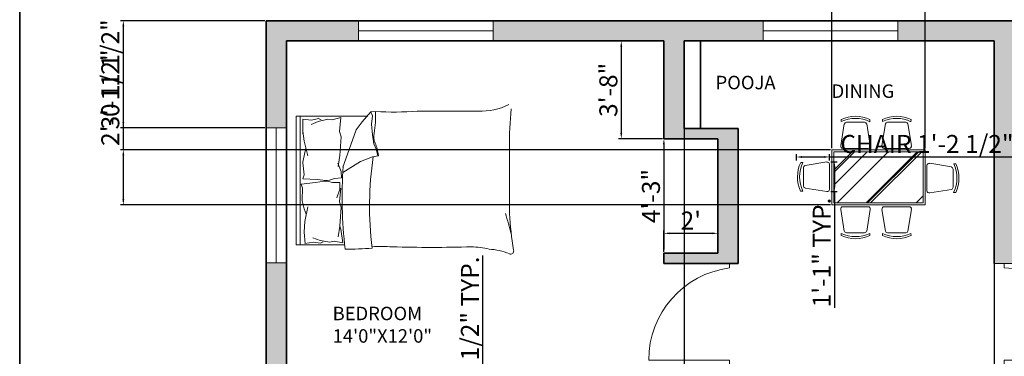
# Model space of a CAD drawing. Units: inches. Extents: x 2257 to 3678, y 834 to 1975.
# Tile 4 of 16: x 2257 to 2696, y 1444 to 1594. Entities that reach past the tile are written whole.
import ezdxf

# ---------------------------------------------------------------- set-up
doc = ezdxf.new("R2010")
doc.units = ezdxf.units.IN
for name, color, linetype, lineweight in [('A-ANNO-DIMS', 2, 'Continuous', 18), ('A-ANNO-TTLB', 7, 'Continuous', 35), ('A-AREA-IDEN', 7, 'Continuous', 18), ('A-DOOR', 3, 'Continuous', 18), ('A-FURN', 8, 'Continuous', 18), ('A-FURN-PATT', 8, 'Continuous', 13), ('A-GLAZ', 4, 'Continuous', 18), ('A-WALL', 7, 'Continuous', 35)]:
    doc.layers.add(name, color=color, linetype=linetype, lineweight=lineweight)
doc.layers.add('A-WALL-PATT', color=251, linetype='Continuous', lineweight=13, true_color=0x636466)
doc.styles.get("Standard").update_dxf_attribs({"font": 'arial.ttf'})
doc.dimstyles.new('ISO-25', dxfattribs={"dimtxt": 8, "dimasz": 2.5, "dimexe": 1.25, "dimexo": 0.625, "dimtad": 1, "dimdec": 0, "dimlunit": 3, "dimtxsty": 'Standard', "dimcen": 2.5, "dimadec": 0, "dimazin": 0, "dimtfac": 1, "dimtdec": 0, "dimtmove": 0, "dimatfit": 3, "dimfxl": 1, "dimarcsym": 0})

# ---------------------------------------------------------------- blocks, each defined once
blk = doc.blocks.new('*D1')
at = {"layer": 'A-ANNO-DIMS', "color": 0, "lineweight": -2, "transparency": 16777216}
for p, q in [((2543.43, 1584.58), (2523.84, 1584.58)), ((2525.09, 1582.08), (2525.09, 1543.58)), ((2543.43, 1541.08), (2523.84, 1541.08))]:
    blk.add_line(p, q, dxfattribs=at)
at = {"layer": 'A-ANNO-DIMS', "color": 0, "transparency": 16777216}
for points in [[(2524.68, 1582.08), (2525.51, 1582.08), (2525.09, 1584.58)], [(2524.68, 1543.58), (2525.51, 1543.58), (2525.09, 1541.08)]]:
    blk.add_solid(points, dxfattribs=at)
at = {"layer": 'Defpoints', "color": 0, "transparency": 16777216}
for p in [(2544.05, 1584.58), (2525.09, 1541.08), (2544.05, 1541.08)]:
    blk.add_point(p, dxfattribs=at)
at = {"layer": 'A-ANNO-DIMS', "color": 0, "transparency": 16777216, "insert": (2520.38, 1562.83), "char_height": 8, "attachment_point": 5, "rotation": 90}
blk.add_mtext('3\'-8"', dxfattribs=at)
blk = doc.blocks.new('*D2')
at = {"layer": 'A-ANNO-DIMS', "color": 0, "lineweight": -2, "transparency": 16777216}
for p, q in [((2544.05, 1538.58), (2544.05, 1492.58)), ((2544.68, 1541.08), (2545.3, 1541.08)), ((2544.68, 1490.08), (2545.3, 1490.08))]:
    blk.add_line(p, q, dxfattribs=at)
at = {"layer": 'A-ANNO-DIMS', "color": 0, "transparency": 16777216}
for points in [[(2543.63, 1538.58), (2544.47, 1538.58), (2544.05, 1541.08)], [(2543.63, 1492.58), (2544.47, 1492.58), (2544.05, 1490.08)]]:
    blk.add_solid(points, dxfattribs=at)
at = {"layer": 'Defpoints', "color": 0, "transparency": 16777216}
for p in [(2544.05, 1541.08), (2544.05, 1490.08), (2544.05, 1490.08)]:
    blk.add_point(p, dxfattribs=at)
at = {"layer": 'A-ANNO-DIMS', "color": 0, "transparency": 16777216, "insert": (2539.34, 1515.58), "char_height": 8, "attachment_point": 5, "rotation": 90}
blk.add_mtext('4\'-3"', dxfattribs=at)
blk = doc.blocks.new('*D3')
at = {"layer": 'A-ANNO-DIMS', "color": 0, "lineweight": -2, "transparency": 16777216}
for p, q in [((2544.05, 1490.7), (2544.05, 1500.22)), ((2546.55, 1498.97), (2565.55, 1498.97)), ((2568.05, 1490.7), (2568.05, 1500.22))]:
    blk.add_line(p, q, dxfattribs=at)
at = {"layer": 'A-ANNO-DIMS', "color": 0, "transparency": 16777216}
for points in [[(2546.55, 1499.38), (2546.55, 1498.55), (2544.05, 1498.97)], [(2565.55, 1499.38), (2565.55, 1498.55), (2568.05, 1498.97)]]:
    blk.add_solid(points, dxfattribs=at)
at = {"layer": 'Defpoints', "color": 0, "transparency": 16777216}
for p in [(2568.05, 1498.97), (2544.05, 1490.08), (2568.05, 1490.08)]:
    blk.add_point(p, dxfattribs=at)
at = {"layer": 'A-ANNO-DIMS', "color": 0, "transparency": 16777216, "insert": (2556.05, 1503.61), "char_height": 8, "attachment_point": 5}
blk.add_mtext("2'", dxfattribs=at)
blk = doc.blocks.new('BED-DOUBLE-PLAN')
for p, q in [((0, 61.46), (31.9, 61.46)), ((0, 4.17), (0, 61.46)), ((1.84, 4.17), (1.84, 61.46)), ((33.26, 63.38), (29.37, 58.94)), ((35.36, 63.48), (33.26, 63.38, 4.64)), ((34.01, 61.54), (33.26, 63.38)), ((33.63, 57.82), (34.01, 61.54)), ((3.07, 60.08), (2.95, 53.6)), ((3.07, 60.08), (6.92, 59.62)), ((9.9, 59.11), (6.69, 57.7)), ((6.92, 59.62), (10, 60.34)), ((14.18, 60.08), (9.9, 59.11)), ((10, 60.34), (11.25, 59.72)), ((16.11, 59.85), (14.18, 60.08)), ((19.87, 60.78), (16.11, 59.85)), ((19.38, 54.63), (19.87, 60.78)), ((29.37, 58.94), (26.77, 55.41)), ((34.01, 53.18), (33.63, 57.82)), ((2.95, 53.6), (3.05, 54.8)), ((3.05, 54.8), (3.68, 50.25)), ((20.05, 52.28), (19.38, 54.63)), ((26.77, 55.41), (24.36, 48.73)), ((34.56, 49.1), (34.01, 53.18)), ((3.68, 50.25), (5.3, 43.75)), ((19.54, 43.87), (20.05, 52.28)), ((24.36, 48.73), (20.84, 38.73)), ((35.68, 46.68), (34.56, 49.1)), ((3.69, 44.52), (3.04, 41.01)), ((4.4, 47), (3.69, 44.52)), ((18.74, 39.04), (19.54, 43.87)), ((36.42, 43.71), (35.68, 46.68)), ((95, 18.06), (95, 47.57)), ((3.04, 41.01), (3.07, 40.62)), ((3.07, 40.62), (3.57, 35.31)), ((20.07, 36.86), (18.53, 40.55)), ((20.84, 36.28), (28.62, 41.3)), ((28.62, 41.3), (34.01, 43.34)), ((34.01, 43.34), (36.42, 43.71)), ((3.57, 35.31), (2.99, 33.54)), ((20.25, 33.92), (20.07, 36.86)), ((2.24, 31.15), (8.66, 31.84)), ((2.94, 29.42), (2.24, 31.15)), ((2.99, 33.54), (9.43, 33.25)), ((8.66, 31.84), (12.47, 32.54)), ((9.43, 33.25), (13.28, 32.79)), ((12.47, 32.54), (14.03, 32.54)), ((13.28, 32.79), (14.84, 32.89)), ((14.03, 32.54), (16.28, 31.84)), ((14.84, 32.89), (17.04, 33.72)), ((16.28, 31.84), (19.5, 31.84)), ((17.04, 33.72), (20.25, 33.92)), ((19.5, 31.84), (19.5, 28.9)), ((2.76, 24.09), (2.94, 29.42)), ((19.5, 28.9), (18.19, 25.13)), ((19.38, 23.24), (19.87, 29.39)), ((2.76, 23.7), (2.76, 24.09)), ((3.63, 20.23), (2.76, 23.7)), ((20.05, 20.89), (19.38, 23.24)), ((4.5, 17.81), (3.63, 20.23)), ((3.98, 14.52), (5.19, 21.1)), ((19.54, 12.48), (20.05, 20.89)), ((3.63, 9.93), (3.98, 14.52)), ((3.61, 9.81), (3.63, 9.93)), ((4, 4.67), (3.61, 9.81)), ((18.74, 7.65), (19.54, 12.48)), ((19.54, 12.48), (19.92, 11.13)), ((19.92, 11.13), (20.79, 5.02)), ((3.98, 4.67), (7.79, 5.36)), ((10.74, 6.06), (7.44, 7.27)), ((7.79, 5.36), (10.91, 4.84)), ((15.07, 5.36), (10.74, 6.06)), ((10.91, 4.84), (12.12, 5.54)), ((16.98, 5.71), (15.07, 5.36)), ((20.79, 5.02), (16.98, 5.71)), ((21.71, 4.17), (0, 4.17))]:
    blk.add_line(p, q)
for centre, radius, start, end in [((82.32, 91.3), 27.65, 267.4714, 296.4681), ((-7.98, 61.53), 43.38, 349.8763, 2.5657), ((43.54, 218.51), 155.25, 266.9791, 273.8365), ((81.31, -5405.34), 5469.02, 90.00217, 90.28689), ((254.49, 49.33), 159.5, 174.4998, 180.6351), ((42.04, 52.44), 7.46, 168.6608, 203.7384), ((1.78, 37.35), 35.55, 10.6617, 19.8806), ((36.49, 43.92), 0.221, 250.2464, 1.1377), ((187.4, 21.29), 154.68, 171.7845, 186.9006), ((218.26, 25.61), 197.77, 176.0865, 186.7821), ((-28.43, -20.65), 127.63, 13.3832, 17.7053), ((240.78, 25.69), 145.97, 182.9958, 189.4091), ((24.09, 102.1), 99.87, 268.7218, 275.604), ((37.37, -200.58), 203.94, 88.4762, 91.0082), ((60.68, 581.23), 578.22, 268.22771, 271.71854), ((77.34, -32.25), 35.53, 76.0648, 88.9113), ((84.25, -25.97), 28.25, 67.9751, 86.652), ((95.57, 1.3), 1.31, 236.1736, 23.4781)]:
    blk.add_arc(centre, radius, start, end)
blk = doc.blocks.new('CHAIR-DINING-PLAN')
for p, q in [((0.97, 14.25), (12.21, 14.25)), ((1.56, 3.41), (0, 13.01)), ((11.61, 3.41), (13.17, 13.01)), ((0.21, 2.36), (0.24, 1.44)), ((10.64, 2.63), (2.54, 2.63)), ((12.98, 1.41), (12.95, 2.39))]:
    blk.add_line(p, q)
for centre, radius, start, end in [((0.97, 13.33), 0.921, 90, 192.3792), ((12.21, 13.33), 0.921, 346.3053, 90), ((6.56, 15.72), 14.78, 244.6873, 295.6189), ((6.65, 14.96), 14.96, 244.649, 295.0455), ((2.54, 3.55), 0.921, 193.6947, 269.5544), ((10.63, 3.55), 0.921, 270.4456, 346.3053)]:
    blk.add_arc(centre, radius, start, end)
blk = doc.blocks.new('WIN-60')
for p, q in [((0, 9), (0, 0)), ((60, 4.5), (60, 9)), ((60, 9), (60, 0)), ((0, 0), (0, 4.5)), ((0, 4.5), (60, 4.5))]:
    blk.add_line(p, q)
blk = doc.blocks.new('WIN-60-SIDE')
for p, q in [((0, 60), (9, 60)), ((9, 60), (4.5, 60)), ((4.5, 60), (4.5, 0)), ((9, 0), (0, 0)), ((4.5, 0), (9, 0))]:
    blk.add_line(p, q)
blk = doc.blocks.new('DOOR-BEDROOM-REAR')
for p, q in [((36, 45), (36, 43)), ((36, 2), (0, 2)), ((36, 0), (36, 2))]:
    blk.add_line(p, q)
blk.add_arc((41.35, 2), 41.35, 97.4306, 180)
blk = doc.blocks.new('DOOR-KITCHEN')
for p, q in [((0, 45), (9, 45)), ((4.5, 45), (4.5, 43)), ((9, 45), (4.5, 45)), ((4.5, 0), (4.5, 2)), ((4.5, 2), (40.5, 2)), ((9, 0), (0, 0))]:
    blk.add_line(p, q)
blk.add_arc((4.5, 6.7), 36.3, 352.5694, 90)
blk = doc.blocks.new('*D49')
at = {"layer": 'A-ANNO-DIMS', "color": 0, "lineweight": -2, "transparency": 16777216}
for p, q in [((2463.54, 1418), (2463.54, 1489.16)), ((2449.61, 1418), (2464.79, 1418)), ((2463.54, 1353.85), (2463.54, 1415.5)), ((2449.61, 1351.35), (2464.79, 1351.35))]:
    blk.add_line(p, q, dxfattribs=at)
at = {"layer": 'A-ANNO-DIMS', "color": 0, "transparency": 16777216}
for points in [[(2463.12, 1415.5), (2463.95, 1415.5), (2463.54, 1418)], [(2463.12, 1353.85), (2463.95, 1353.85), (2463.54, 1351.35)]]:
    blk.add_solid(points, dxfattribs=at)
at = {"layer": 'Defpoints', "color": 0, "transparency": 16777216}
for p in [(2448.99, 1418), (2463.54, 1418), (2448.99, 1351.35)]:
    blk.add_point(p, dxfattribs=at)
at = {"layer": 'A-ANNO-DIMS', "color": 0, "transparency": 16777216, "insert": (2458.78, 1454.83), "char_height": 8, "attachment_point": 5, "rotation": 90}
blk.add_mtext('5\'-6 1/2" TYP.', dxfattribs=at)
blk = doc.blocks.new('*D50')
at = {"layer": 'A-ANNO-DIMS', "color": 0, "lineweight": -2, "transparency": 16777216}
for p, q in [((2603.02, 1531.36), (2603.02, 1534.2)), ((2617.76, 1531.36), (2617.76, 1534.2)), ((2605.52, 1532.95), (2615.26, 1532.95)), ((2617.76, 1532.95), (2726.7, 1532.95))]:
    blk.add_line(p, q, dxfattribs=at)
at = {"layer": 'A-ANNO-DIMS', "color": 0, "transparency": 16777216}
for points in [[(2605.52, 1533.37), (2605.52, 1532.53), (2603.02, 1532.95)], [(2615.26, 1533.37), (2615.26, 1532.53), (2617.76, 1532.95)]]:
    blk.add_solid(points, dxfattribs=at)
at = {"layer": 'Defpoints', "color": 0, "transparency": 16777216}
for p in [(2603.02, 1530.74), (2617.76, 1532.95), (2617.76, 1530.74)]:
    blk.add_point(p, dxfattribs=at)
at = {"layer": 'A-ANNO-DIMS', "color": 0, "transparency": 16777216, "insert": (2673.48, 1537.71), "char_height": 8, "attachment_point": 5}
blk.add_mtext('CHAIR 1\'-2 1/2" TYP.', dxfattribs=at)
blk = doc.blocks.new('*D51')
at = {"layer": 'A-ANNO-DIMS', "color": 0, "lineweight": -2, "transparency": 16777216}
for p, q in [((2618.38, 1530.74), (2621.22, 1530.74)), ((2619.97, 1528.24), (2619.97, 1520.07)), ((2618.38, 1517.57), (2621.22, 1517.57)), ((2619.97, 1517.57), (2619.97, 1465.81))]:
    blk.add_line(p, q, dxfattribs=at)
at = {"layer": 'A-ANNO-DIMS', "color": 0, "transparency": 16777216}
for points in [[(2619.55, 1528.24), (2620.39, 1528.24), (2619.97, 1530.74)], [(2619.55, 1520.07), (2620.39, 1520.07), (2619.97, 1517.57)]]:
    blk.add_solid(points, dxfattribs=at)
at = {"layer": 'Defpoints', "color": 0, "transparency": 16777216}
for p in [(2617.76, 1530.74), (2617.76, 1517.57), (2619.97, 1517.57)]:
    blk.add_point(p, dxfattribs=at)
at = {"layer": 'A-ANNO-DIMS', "color": 0, "transparency": 16777216, "insert": (2615.32, 1490.44), "char_height": 8, "attachment_point": 5, "rotation": 90}
blk.add_mtext('1\'-1" TYP.', dxfattribs=at)
blk = doc.blocks.new('*D106')
at = {"layer": 'A-ANNO-DIMS', "color": 0, "lineweight": -2, "transparency": 16777216}
for p, q in [((2553.05, 1583.95), (2553.05, 894.3)), ((2691.05, 1583.95), (2691.05, 894.3)), ((2555.55, 895.55), (2688.55, 895.55))]:
    blk.add_line(p, q, dxfattribs=at)
at = {"layer": 'A-ANNO-DIMS', "color": 0, "transparency": 16777216}
for points in [[(2555.55, 895.97), (2555.55, 895.14), (2553.05, 895.55)], [(2688.55, 895.97), (2688.55, 895.14), (2691.05, 895.55)]]:
    blk.add_solid(points, dxfattribs=at)
at = {"layer": 'Defpoints', "color": 0, "transparency": 16777216}
for p in [(2553.05, 1584.58), (2691.05, 1584.58), (2691.05, 895.55)]:
    blk.add_point(p, dxfattribs=at)
at = {"layer": 'A-ANNO-DIMS', "color": 0, "transparency": 16777216, "insert": (2622.05, 900.26), "char_height": 8, "attachment_point": 5}
blk.add_mtext('11\'-6"', dxfattribs=at)
blk = doc.blocks.new('*D111')
at = {"layer": 'A-ANNO-DIMS', "color": 0, "lineweight": -2, "transparency": 16777216}
for p, q in [((2366.43, 1593.58), (2302.25, 1593.58)), ((2303.5, 1548.39), (2303.5, 1591.08)), ((2366.43, 1545.89), (2302.25, 1545.89))]:
    blk.add_line(p, q, dxfattribs=at)
at = {"layer": 'A-ANNO-DIMS', "color": 0, "transparency": 16777216}
for points in [[(2303.08, 1591.08), (2303.92, 1591.08), (2303.5, 1593.58)], [(2303.08, 1548.39), (2303.92, 1548.39), (2303.5, 1545.89)]]:
    blk.add_solid(points, dxfattribs=at)
at = {"layer": 'Defpoints', "color": 0, "transparency": 16777216}
for p in [(2303.5, 1593.58), (2367.05, 1593.58), (2367.05, 1545.89)]:
    blk.add_point(p, dxfattribs=at)
at = {"layer": 'A-ANNO-DIMS', "color": 0, "transparency": 16777216, "insert": (2298.74, 1569.73), "char_height": 8, "attachment_point": 5, "rotation": 90}
blk.add_mtext('3\'-11 1/2"', dxfattribs=at)
blk = doc.blocks.new('*D115')
at = {"layer": 'A-ANNO-DIMS', "color": 0, "lineweight": -2, "transparency": 16777216}
for p, q in [((2618.78, 1536.81), (2618.78, 1628.38)), ((2621.28, 1627.13), (2657.85, 1627.13)), ((2660.35, 1536.81), (2660.35, 1628.38))]:
    blk.add_line(p, q, dxfattribs=at)
at = {"layer": 'A-ANNO-DIMS', "color": 0, "transparency": 16777216}
for points in [[(2621.28, 1627.54), (2621.28, 1626.71), (2618.78, 1627.13)], [(2657.85, 1627.54), (2657.85, 1626.71), (2660.35, 1627.13)]]:
    blk.add_solid(points, dxfattribs=at)
at = {"layer": 'Defpoints', "color": 0, "transparency": 16777216}
for p in [(2660.35, 1627.13), (2618.78, 1536.18), (2660.35, 1536.18)]:
    blk.add_point(p, dxfattribs=at)
at = {"layer": 'A-ANNO-DIMS', "color": 0, "transparency": 16777216, "insert": (2639.56, 1631.89), "char_height": 8, "attachment_point": 5}
blk.add_mtext('3\'-5 1/2"', dxfattribs=at)
blk = doc.blocks.new('*D116')
at = {"layer": 'A-ANNO-DIMS', "color": 0, "lineweight": -2, "transparency": 16777216}
for p, q in [((2303.5, 1536.18), (2303.5, 1579.98)), ((2618.15, 1536.18), (2302.25, 1536.18)), ((2303.5, 1514.1), (2303.5, 1533.68)), ((2618.15, 1511.6), (2302.25, 1511.6))]:
    blk.add_line(p, q, dxfattribs=at)
at = {"layer": 'A-ANNO-DIMS', "color": 0, "transparency": 16777216}
for points in [[(2303.08, 1533.68), (2303.92, 1533.68), (2303.5, 1536.18)], [(2303.08, 1514.1), (2303.92, 1514.1), (2303.5, 1511.6)]]:
    blk.add_solid(points, dxfattribs=at)
at = {"layer": 'Defpoints', "color": 0, "transparency": 16777216}
for p in [(2303.5, 1536.18), (2618.78, 1536.18), (2618.78, 1511.6)]:
    blk.add_point(p, dxfattribs=at)
at = {"layer": 'A-ANNO-DIMS', "color": 0, "transparency": 16777216, "insert": (2298.74, 1559.33), "char_height": 8, "attachment_point": 5, "rotation": 90}
blk.add_mtext('2\'-0 1/2"', dxfattribs=at)

msp = doc.modelspace()

# ---------------------------------------------------------------- hatches: boundary and pattern name
at = {"layer": 'A-FURN-PATT'}
h = msp.add_hatch(dxfattribs=at)
h.set_pattern_fill('AR-RROOF', color=256, scale=0.620125, angle=45, style=0)
h.set_pattern_definition([(45, (1777.685, 1859.039), (13.36532, 35.64084), [236.2676, -31.5024, 78.7559, -15.7512]), (45, (1786.93, 1879.42), (-25.951, 3.67546), [47.2535, -5.1979, 94.507, -11.8134]), (45, (1773.787, 1874.074), (50.45407, 65.37867), [126.0094, -22.0516, 63.0047, -15.7512])])
h.paths.add_polyline_path([(2619.71, 1535.25), (2619.71, 1512.53), (2659.42, 1512.53), (2659.42, 1535.25)])
at = {"layer": 'A-WALL-PATT'}
h = msp.add_hatch(color=256, dxfattribs=at)
h.dxf.hatch_style = 1
h.paths.add_polyline_path([(2736.02, 1589.08), (2736.02, 1593.58), (2691.05, 1593.58), (2648.2, 1593.58), (2648.2, 1584.58), (2691.05, 1584.58), (2691.05, 1485.58), (2700.05, 1485.58), (2700.05, 1584.58), (2736.02, 1584.58)])
h.paths.add_polyline_path([(2835.05, 1593.58), (2796.02, 1593.58), (2796.02, 1584.58), (2826.05, 1584.58), (2826.05, 1440.58), (2835.05, 1440.58)])
h.paths.add_polyline_path([(2865.05, 1440.58), (2826.05, 1440.58), (2700.05, 1440.58), (2691.05, 1440.58), (2691.05, 1431.58), (2691.05, 1284.58), (2700.05, 1284.58), (2700.05, 1431.58), (2826.05, 1431.58), (2856.05, 1431.58), (2856.05, 1395.2), (2865.05, 1395.2), (2865.05, 1431.58)])
h.paths.add_polyline_path([(2865.05, 1335.2), (2856.05, 1335.2), (2856.05, 1293.58), (2741.94, 1293.58), (2741.94, 1289.08), (2741.94, 1284.58), (2865.05, 1284.58)], flags=17)
h.paths.add_polyline_path([(2865.05, 1172.08), (2856.05, 1172.08), (2741.94, 1172.08), (2741.94, 1163.08), (2856.05, 1163.08), (2856.05, 1133.53), (2865.05, 1133.53)])
h.paths.add_polyline_path([(2865.05, 1073.53), (2856.05, 1073.53), (2856.05, 1019.08), (2795.28, 1019.08), (2795.28, 1010.08), (2865.05, 1010.08)])
h.paths.add_polyline_path([(2735.28, 1014.58), (2735.28, 1019.08), (2700.05, 1019.08), (2700.05, 1026.35), (2695.55, 1026.35), (2691.05, 1026.35), (2691.05, 1010.08), (2735.28, 1010.08)])
h.paths.add_polyline_path([(2700.05, 1163.08), (2700.05, 1172.08), (2691.05, 1172.08), (2685.7, 1172.08), (2685.7, 1163.08), (2691.05, 1163.08), (2691.05, 1058.19), (2700.05, 1058.19)])
h.paths.add_polyline_path([(2707.1, 1172.08), (2700.05, 1172.08), (2700.05, 1163.08), (2707.1, 1163.08)])
h.paths.add_polyline_path([(2685.7, 1172.08), (2678.22, 1172.08), (2678.22, 1163.08), (2685.7, 1163.08)])
h.paths.add_polyline_path([(2654.22, 1172.08), (2648.96, 1172.08), (2648.96, 1163.08), (2654.22, 1163.08), (2654.22, 1167.58)])
h.paths.add_polyline_path([(2553.05, 1163.08), (2558.66, 1163.08), (2558.66, 1172.08), (2544.05, 1172.08), (2544.05, 1163.08), (2544.05, 1058.19), (2553.05, 1058.19)])
h.paths.add_polyline_path([(2568.8, 1167.58), (2568.8, 1172.08), (2558.66, 1172.08), (2558.66, 1163.08), (2568.8, 1163.08)])
h.paths.add_polyline_path([(2596.82, 1172.08), (2592.8, 1172.08), (2592.8, 1163.08), (2596.82, 1163.08)])
h.paths.add_polyline_path([(2553.05, 1019.08), (2553.05, 1026.35), (2548.55, 1026.35), (2544.05, 1026.35), (2544.05, 1019.08), (2476.8, 1019.08), (2476.8, 1010.08), (2553.05, 1010.08)])
h.paths.add_polyline_path([(2376.05, 1163.08), (2502.05, 1163.08), (2502.05, 1172.08), (2446.55, 1172.08), (2446.55, 1195.52), (2446.55, 1215.32), (2442.05, 1215.32), (2442.05, 1195.52), (2442.05, 1172.08), (2412.05, 1172.08), (2412.05, 1167.58), (2376.05, 1167.58), (2376.05, 1172.08), (2376.05, 1201.28), (2367.05, 1201.28), (2367.05, 1172.08), (2367.05, 1123.86), (2376.05, 1123.86)])
h.paths.add_polyline_path([(2577.05, 1440.58), (2376.05, 1440.58), (2376.05, 1485.89), (2367.05, 1485.89), (2367.05, 1440.58), (2337.05, 1440.58), (2337.05, 1403.59), (2346.05, 1403.59), (2346.05, 1431.58), (2493.05, 1431.58), (2493.05, 1293.58), (2484.41, 1293.58), (2484.41, 1284.58), (2502.05, 1284.58), (2502.05, 1431.58), (2577.05, 1431.58)])
h.paths.add_polyline_path([(2346.05, 1343.59), (2337.05, 1343.59), (2337.05, 1284.58), (2448.12, 1284.58), (2448.12, 1289.08), (2448.12, 1293.58), (2346.05, 1293.58)], flags=17)
h.paths.add_polyline_path([(2376.05, 1244.08), (2446.55, 1244.08), (2446.55, 1248.58), (2367.05, 1248.58), (2367.05, 1225.28), (2375.64, 1225.28), (2375.64, 1228.02), (2376.05, 1228.02)])
h.paths.add_polyline_path([(2588.2, 1589.08), (2588.2, 1593.58), (2468.1, 1593.58), (2468.1, 1584.58), (2544.05, 1584.58), (2544.05, 1541.08), (2568.05, 1541.08), (2568.05, 1490.08), (2544.05, 1490.08), (2544.05, 1485.58), (2577.05, 1485.58), (2577.05, 1545.58), (2553.05, 1545.58), (2553.05, 1584.58), (2588.2, 1584.58)])
h.paths.add_polyline_path([(2376.05, 1584.58), (2408.1, 1584.58), (2408.1, 1589.08), (2408.1, 1593.58), (2367.05, 1593.58), (2367.05, 1545.89), (2376.05, 1545.89)])
h.paths.add_polyline_path([(2376.05, 1063.86), (2367.05, 1063.86), (2367.05, 1019.08), (2367.05, 1010.08), (2416.8, 1010.08), (2416.8, 1014.58), (2416.8, 1019.08), (2376.05, 1019.08)])

# ---------------------------------------------------------------- linework, layer by layer
at = {"layer": 'A-ANNO-TTLB'}
msp.add_lwpolyline([(2257.38, 1974.9), (3677.96, 1974.9), (3677.96, 849.42), (2257.38, 849.42)], close=True, dxfattribs=at)
at = {"layer": 'A-FURN'}
for p, q in [((2671.98, 1528.57), (2662.37, 1530.13)), ((2673.03, 1529.92), (2673.94, 1529.89)), ((2661.13, 1529.16), (2661.13, 1517.92)), ((2672.75, 1519.49), (2672.75, 1527.59)), ((2671.98, 1518.52), (2662.37, 1516.96)), ((2673.98, 1517.14), (2672.99, 1517.18))]:
    msp.add_line(p, q, dxfattribs=at)
for points in [[(2618.78, 1536.18), (2660.35, 1536.18), (2660.35, 1511.6), (2618.78, 1511.6)], [(2619.71, 1535.25), (2659.42, 1535.25), (2659.42, 1512.53), (2619.71, 1512.53)]]:
    msp.add_lwpolyline(points, close=True, dxfattribs=at)
for centre, radius, start, end in [((2662.05, 1529.16), 0.921, 77.6208, 180), ((2659.67, 1523.57), 14.78, 334.3811, 25.3127), ((2660.42, 1523.48), 14.96, 334.9545, 25.351), ((2671.83, 1527.59), 0.921, 0.4456, 76.3053), ((2662.17, 1517.98), 1.04, 183.2545, 281.1166), ((2671.68, 1519.55), 1.08, 286.0311, 356.7526)]:
    msp.add_arc(centre, radius, start, end, dxfattribs=at)
at = {"layer": 'A-WALL'}
for p, q in [((2367.05, 1593.58), (2367.05, 1440.58)), ((2367.05, 1593.58), (2835.05, 1593.58)), ((2367.05, 1593.58), (2648.2, 1593.58)), ((2691.05, 1593.58), (2835.05, 1593.58)), ((2376.05, 1584.58), (2544.05, 1584.58)), ((2376.05, 1584.58), (2376.05, 1440.58)), ((2544.05, 1584.58), (2544.05, 1541.08)), ((2553.05, 1584.58), (2553.05, 1545.58)), ((2553.05, 1584.58), (2553.05, 1545.58)), ((2553.05, 1584.58), (2691.05, 1584.58)), ((2560.36, 1545.58), (2560.36, 1584.58)), ((2691.05, 1584.58), (2691.05, 1485.58)), ((2553.05, 1545.58), (2577.05, 1545.58)), ((2577.05, 1545.58), (2577.05, 1485.58)), ((2568.05, 1541.08), (2544.05, 1541.08)), ((2568.05, 1490.08), (2568.05, 1541.08)), ((2544.05, 1485.58), (2544.05, 1490.08)), ((2544.05, 1490.08), (2568.05, 1490.08)), ((2544.05, 1490.08), (2544.05, 1485.58)), ((2577.05, 1485.58), (2544.05, 1485.58))]:
    msp.add_line(p, q, dxfattribs=at)

# ---------------------------------------------------------------- block references
at = {"layer": 'A-DOOR'}
for name, p in [('DOOR-BEDROOM-REAR', (2537.29, 1440.58)), ('DOOR-KITCHEN', (2691.05, 1440.58))]:
    msp.add_blockref(name, p, dxfattribs=at)
at = {"layer": 'A-FURN'}
for name, p in [('BED-DOUBLE-PLAN', (2380.36, 1489.7)), ('CHAIR-DINING-PLAN', (2622.74, 1496.57)), ('CHAIR-DINING-PLAN', (2641.07, 1496.57))]:
    msp.add_blockref(name, p, dxfattribs=at)
at = {"layer": 'A-FURN', "extrusion": (0, 0, -1), "zscale": -1, "rotation": 180}
for p in [(-2622.74, 1551.05), (-2641.07, 1551.05)]:
    msp.add_blockref('CHAIR-DINING-PLAN', p, dxfattribs=at)
at = {"layer": 'A-FURN', "rotation": 269.999999943256}
msp.add_blockref('CHAIR-DINING-PLAN', (2603.5, 1530.74), dxfattribs=at)
at = {"layer": 'A-GLAZ'}
for name, p in [('WIN-60', (2408.1, 1584.58)), ('WIN-60', (2588.2, 1584.58)), ('WIN-60-SIDE', (2367.05, 1485.89))]:
    msp.add_blockref(name, p, dxfattribs=at)

# ---------------------------------------------------------------- texts
at = {"layer": 'A-AREA-IDEN', "char_height": 6, "attachment_point": 1}
for s, width, insert in [('POOJA', 24.6829, (2567.07, 1569.08)), ('DINING', 132.26, (2618.69, 1565.25)), ('BEDROOM\\P14\'0"X12\'0"', 262.7298, (2396.64, 1466.29))]:
    msp.add_mtext_dynamic_manual_height_columns(s, width=width, gutter_width=12.5, heights=[0], dxfattribs=dict(at, insert=insert))

# ---------------------------------------------------------------- dimensions: what is measured, and where the dimension line sits
at = {"layer": 'A-ANNO-DIMS'}
for base, p1, p2, override, picture, middle in [((2660.35, 1627.13), (2618.78, 1536.18), (2660.35, 1536.18), {"dimdec": 1, "dimlfac": 1, "dimrnd": 0, "dimzin": 1, "dimdsep": 46, "dimlunit": 4, "dimfrac": 2}, '*D115', (2639.56, 1631.89)), ((2691.05, 895.55), (2553.05, 1584.58), (2691.05, 1584.58), {"dimdec": 1, "dimlfac": 1, "dimrnd": 0, "dimzin": 1, "dimdsep": 46, "dimlunit": 4, "dimfrac": 2}, '*D106', (2622.05, 900.26)), ((2568.05, 1498.97), (2544.05, 1490.08), (2568.05, 1490.08), {"dimclrd": 0, "dimclre": 0, "dimclrt": 0}, '*D3', (2556.05, 1503.61))]:
    dim = msp.add_linear_dim(base=base, p1=p1, p2=p2, dimstyle='ISO-25', override=override, dxfattribs=at)
    dim.commit()
    dim.dimension.update_dxf_attribs({"geometry": picture, "text_midpoint": middle})
for base, p1, p2, override, picture, middle in [((2303.5, 1593.58), (2367.05, 1545.89), (2367.05, 1593.58), {"dimdec": 1, "dimlfac": 1, "dimrnd": 0, "dimzin": 1, "dimdsep": 46, "dimlunit": 4, "dimfrac": 2}, '*D111', (2298.74, 1569.73)), ((2525.09329705, 1541.07694214), (2544.05094479, 1584.57694214), (2544.05094479, 1541.07694214), {"dimclrd": 0, "dimclre": 0, "dimclrt": 0}, '*D1', (2520.38098464, 1562.82694214)), ((2303.5, 1536.18), (2618.78, 1511.6), (2618.78, 1536.18), {"dimdec": 1, "dimlfac": 1, "dimrnd": 0, "dimzin": 1, "dimdsep": 46, "dimlunit": 4, "dimfrac": 2}, '*D116', (2298.74, 1559.33)), ((2544.05, 1490.08), (2544.05, 1541.08), (2544.05, 1490.08), {"dimclrd": 0, "dimclre": 0, "dimclrt": 0}, '*D2', (2539.34, 1515.58))]:
    dim = msp.add_linear_dim(base=base, p1=p1, p2=p2, angle=90, dimstyle='ISO-25', override=override, dxfattribs=at)
    dim.commit()
    dim.dimension.update_dxf_attribs({"geometry": picture, "text_midpoint": middle})
for base, p1, p2, angle, text, picture, middle in [((2617.76, 1532.95), (2603.02, 1530.74), (2617.76, 1530.74), 360, 'CHAIR <> TYP.', '*D50', (2673.48, 1537.71)), ((2619.97, 1517.57), (2617.76, 1530.74), (2617.76, 1517.57), 270, '<> TYP.', '*D51', (2615.32, 1490.44)), ((2463.5382, 1418.0044), (2448.9884, 1351.3529), (2448.9884, 1418.0044), 90, '<> TYP.', '*D49', (2458.7768, 1454.832))]:
    dim = msp.add_linear_dim(base=base, p1=p1, p2=p2, angle=angle, text=text, dimstyle='ISO-25', override={"dimdec": 1, "dimlfac": 1, "dimrnd": 0, "dimzin": 1, "dimdsep": 46, "dimlunit": 4, "dimfrac": 2}, dxfattribs=at)
    dim.commit()
    dim.dimension.update_dxf_attribs({"geometry": picture, "text_midpoint": middle})

doc.saveas('drawing.dxf')
